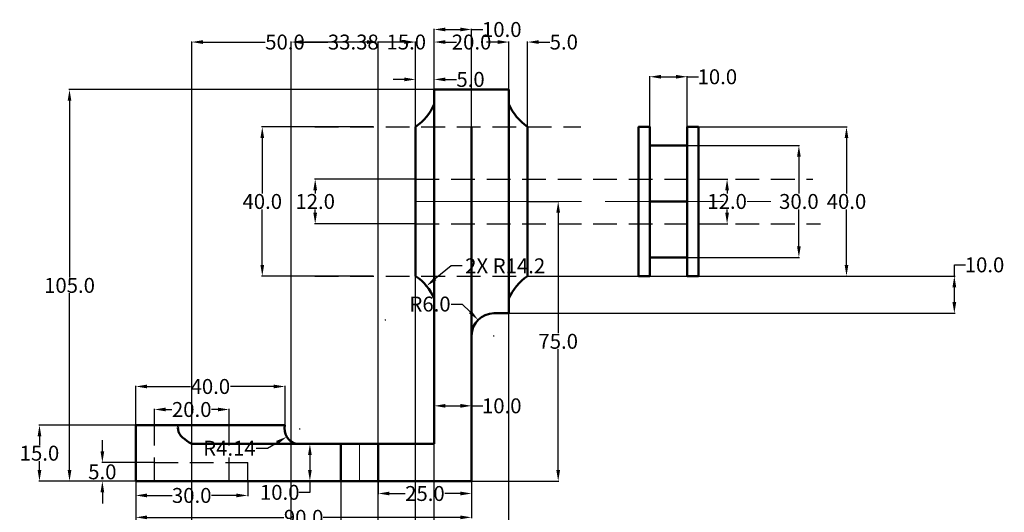
# Model space of a CAD drawing. Units: inches. Extents: x 846 to 1110, y 407 to 675.
# Tile 2 of 2: x 846 to 1110, y 542 to 675. Entities that reach past the tile are written whole.
import ezdxf

# ---------------------------------------------------------------- set-up
doc = ezdxf.new("R2010")
doc.units = ezdxf.units.IN
doc.header["$MEASUREMENT"] = 0
doc.linetypes.add('CENTER', pattern=[50.8, 31.75, -6.35, 6.35, -6.35])
doc.linetypes.add('HIDDEN', pattern=[9.525, 6.35, -3.175])
for name, color, linetype, lineweight in [('M-CNTR', 1, 'CENTER', 18), ('M-DIMS', 2, 'Continuous', 25), ('M-HIDN', 30, 'HIDDEN', 25), ('M-OUTL', 7, 'Continuous', 50)]:
    doc.layers.add(name, color=color, linetype=linetype, lineweight=lineweight)
doc.styles.get("Standard").update_dxf_attribs({"font": 'arial.ttf'})
doc.dimstyles.get("Standard").update_dxf_attribs({"dimtxt": 4, "dimasz": 3, "dimexe": 0.18, "dimexo": 0.0625, "dimgap": 0.09, "dimtad": 0, "dimtih": 1, "dimtoh": 1, "dimdec": 1, "dimzin": 0, "dimdsep": 46, "dimtxsty": 'Standard', "dimcen": 0.09, "dimadec": 0, "dimazin": 0, "dimtfac": 1, "dimtdec": 1, "dimtofl": 0, "dimtmove": 0, "dimatfit": 3, "dimfxl": 1, "dimtolj": 1, "dimtzin": 0, "dimarcsym": 0})

# ---------------------------------------------------------------- blocks, each defined once
blk = doc.blocks.new('*D1')
at = {"layer": 'Defpoints', "color": 0, "transparency": 16777216}
for p in [(902.2, 570.05), (882.2, 565.83), (902.2, 565.83)]:
    blk.add_point(p, dxfattribs=at)
at = {"layer": 'M-DIMS', "color": 0, "lineweight": -2, "transparency": 16777216}
for p, q in [((882.2, 565.9), (882.2, 570.23)), ((885.2, 570.05), (886.88, 570.05)), ((899.2, 570.05), (897.51, 570.05)), ((902.2, 565.9), (902.2, 570.23))]:
    blk.add_line(p, q, dxfattribs=at)
at = {"layer": 'M-DIMS', "color": 0, "transparency": 16777216}
for points in [[(885.2, 570.55), (885.2, 569.55), (882.2, 570.05)], [(899.2, 570.55), (899.2, 569.55), (902.2, 570.05)]]:
    blk.add_solid(points, dxfattribs=at)
at = {"layer": 'M-DIMS', "color": 0, "transparency": 16777216, "insert": (892.2, 570.05), "char_height": 4, "attachment_point": 5}
blk.add_mtext('\\A1;20.0', dxfattribs=at)
blk = doc.blocks.new('*D2')
at = {"layer": 'Defpoints', "color": 0, "transparency": 16777216}
for p in [(917.2, 576.22), (877.2, 565.83), (917.2, 565.83)]:
    blk.add_point(p, dxfattribs=at)
at = {"layer": 'M-DIMS', "color": 0, "lineweight": -2, "transparency": 16777216}
for p, q in [((877.2, 565.9), (877.2, 576.4)), ((880.2, 576.22), (891.84, 576.22)), ((914.2, 576.22), (902.56, 576.22)), ((917.2, 565.9), (917.2, 576.4))]:
    blk.add_line(p, q, dxfattribs=at)
at = {"layer": 'M-DIMS', "color": 0, "transparency": 16777216}
for points in [[(880.2, 576.72), (880.2, 575.72), (877.2, 576.22)], [(914.2, 576.72), (914.2, 575.72), (917.2, 576.22)]]:
    blk.add_solid(points, dxfattribs=at)
at = {"layer": 'M-DIMS', "color": 0, "transparency": 16777216, "insert": (897.2, 576.22), "char_height": 4, "attachment_point": 5}
blk.add_mtext('\\A1;40.0', dxfattribs=at)
blk = doc.blocks.new('*D3')
at = {"layer": 'Defpoints', "color": 0, "transparency": 16777216}
for p in [(877.2, 565.83), (851.4, 550.83), (877.2, 550.83)]:
    blk.add_point(p, dxfattribs=at)
at = {"layer": 'M-DIMS', "color": 0, "lineweight": -2, "transparency": 16777216}
for p, q in [((877.13, 565.83), (851.22, 565.83)), ((851.4, 562.83), (851.4, 560.47)), ((851.4, 553.83), (851.4, 556.2)), ((877.13, 550.83), (851.22, 550.83))]:
    blk.add_line(p, q, dxfattribs=at)
at = {"layer": 'M-DIMS', "color": 0, "transparency": 16777216}
for points in [[(850.9, 562.83), (851.9, 562.83), (851.4, 565.83)], [(850.9, 553.83), (851.9, 553.83), (851.4, 550.83)]]:
    blk.add_solid(points, dxfattribs=at)
at = {"layer": 'M-DIMS', "color": 0, "transparency": 16777216, "insert": (851.4, 558.33), "char_height": 4, "attachment_point": 5}
blk.add_mtext('\\A1;15.0', dxfattribs=at)
blk = doc.blocks.new('*D4')
at = {"layer": 'Defpoints', "color": 0, "transparency": 16777216}
for p in [(882.2, 555.83), (868.25, 550.83), (882.2, 550.83)]:
    blk.add_point(p, dxfattribs=at)
at = {"layer": 'M-DIMS', "color": 0, "lineweight": -2, "transparency": 16777216}
for p, q in [((868.25, 558.83), (868.25, 561.83)), ((882.13, 555.83), (868.07, 555.83)), ((882.13, 550.83), (868.07, 550.83)), ((868.25, 547.83), (868.25, 544.83))]:
    blk.add_line(p, q, dxfattribs=at)
at = {"layer": 'M-DIMS', "color": 0, "transparency": 16777216}
for points in [[(867.75, 558.83), (868.75, 558.83), (868.25, 555.83)], [(867.75, 547.83), (868.75, 547.83), (868.25, 550.83)]]:
    blk.add_solid(points, dxfattribs=at)
at = {"layer": 'M-DIMS', "color": 0, "transparency": 16777216, "insert": (868.25, 553.33), "char_height": 4, "attachment_point": 5}
blk.add_mtext('\\A1;5.0', dxfattribs=at)
blk = doc.blocks.new('*D5')
at = {"layer": 'Defpoints', "color": 0, "transparency": 16777216}
for p in [(877.2, 550.83), (907.2, 550.83), (907.2, 547)]:
    blk.add_point(p, dxfattribs=at)
at = {"layer": 'M-DIMS', "color": 0, "lineweight": -2, "transparency": 16777216}
for p, q in [((877.2, 550.77), (877.2, 546.82)), ((907.2, 550.77), (907.2, 546.82)), ((880.2, 547), (886.92, 547)), ((904.2, 547), (897.47, 547))]:
    blk.add_line(p, q, dxfattribs=at)
at = {"layer": 'M-DIMS', "color": 0, "transparency": 16777216}
for points in [[(880.2, 547.5), (880.2, 546.5), (877.2, 547)], [(904.2, 547.5), (904.2, 546.5), (907.2, 547)]]:
    blk.add_solid(points, dxfattribs=at)
at = {"layer": 'M-DIMS', "color": 0, "transparency": 16777216, "insert": (892.2, 547), "char_height": 4, "attachment_point": 5}
blk.add_mtext('\\A1;30.0', dxfattribs=at)
blk = doc.blocks.new('*D6')
at = {"layer": 'Defpoints', "color": 0, "transparency": 16777216}
for p in [(877.2, 550.83), (967.2, 550.83), (967.2, 541.12)]:
    blk.add_point(p, dxfattribs=at)
at = {"layer": 'M-DIMS', "color": 0, "lineweight": -2, "transparency": 16777216}
for p, q in [((877.2, 550.77), (877.2, 540.94)), ((967.2, 550.77), (967.2, 540.94)), ((880.2, 541.12), (916.92, 541.12)), ((964.2, 541.12), (927.47, 541.12))]:
    blk.add_line(p, q, dxfattribs=at)
at = {"layer": 'M-DIMS', "color": 0, "transparency": 16777216}
for points in [[(880.2, 541.62), (880.2, 540.62), (877.2, 541.12)], [(964.2, 541.62), (964.2, 540.62), (967.2, 541.12)]]:
    blk.add_solid(points, dxfattribs=at)
at = {"layer": 'M-DIMS', "color": 0, "transparency": 16777216, "insert": (922.2, 541.12), "char_height": 4, "attachment_point": 5}
blk.add_mtext('\\A1;90.0', dxfattribs=at)
blk = doc.blocks.new('*D7')
at = {"layer": 'Defpoints', "color": 0, "transparency": 16777216}
for p in [(924.94, 560.83), (923.87, 550.83), (924.94, 550.83)]:
    blk.add_point(p, dxfattribs=at)
at = {"layer": 'M-DIMS', "color": 0, "lineweight": -2, "transparency": 16777216}
for p, q in [((924.87, 560.83), (923.69, 560.83)), ((923.87, 557.83), (923.87, 553.83)), ((924.87, 550.83), (923.69, 550.83)), ((923.87, 550.83), (923.87, 547.83)), ((923.87, 547.83), (920.87, 547.83))]:
    blk.add_line(p, q, dxfattribs=at)
at = {"layer": 'M-DIMS', "color": 0, "transparency": 16777216}
for points in [[(923.37, 557.83), (924.37, 557.83), (923.87, 560.83)], [(923.37, 553.83), (924.37, 553.83), (923.87, 550.83)]]:
    blk.add_solid(points, dxfattribs=at)
at = {"layer": 'M-DIMS', "color": 0, "transparency": 16777216, "insert": (915.78, 547.83), "char_height": 4, "attachment_point": 5}
blk.add_mtext('\\A1;10.0', dxfattribs=at)
blk = doc.blocks.new('*D8')
at = {"layer": 'Defpoints', "color": 0, "transparency": 16777216}
for p in [(942.2, 550.83), (967.2, 550.83), (967.2, 547.52)]:
    blk.add_point(p, dxfattribs=at)
at = {"layer": 'M-DIMS', "color": 0, "lineweight": -2, "transparency": 16777216}
for p, q in [((942.2, 550.77), (942.2, 547.34)), ((967.2, 550.77), (967.2, 547.34)), ((945.2, 547.52), (949.38, 547.52)), ((964.2, 547.52), (960.01, 547.52))]:
    blk.add_line(p, q, dxfattribs=at)
at = {"layer": 'M-DIMS', "color": 0, "transparency": 16777216}
for points in [[(945.2, 548.02), (945.2, 547.02), (942.2, 547.52)], [(964.2, 548.02), (964.2, 547.02), (967.2, 547.52)]]:
    blk.add_solid(points, dxfattribs=at)
at = {"layer": 'M-DIMS', "color": 0, "transparency": 16777216, "insert": (954.7, 547.52), "char_height": 4, "attachment_point": 5}
blk.add_mtext('\\A1;25.0', dxfattribs=at)
blk = doc.blocks.new('*D9')
at = {"layer": 'Defpoints', "color": 0, "transparency": 16777216}
for p in [(940.93, 645.83), (911.11, 605.83), (940.93, 605.83)]:
    blk.add_point(p, dxfattribs=at)
at = {"layer": 'M-DIMS', "color": 0, "lineweight": -2, "transparency": 16777216}
for p, q in [((940.87, 645.83), (910.93, 645.83)), ((911.11, 642.83), (911.11, 627.97)), ((911.11, 608.83), (911.11, 623.7)), ((940.87, 605.83), (910.93, 605.83))]:
    blk.add_line(p, q, dxfattribs=at)
at = {"layer": 'M-DIMS', "color": 0, "transparency": 16777216}
for points in [[(910.61, 642.83), (911.61, 642.83), (911.11, 645.83)], [(910.61, 608.83), (911.61, 608.83), (911.11, 605.83)]]:
    blk.add_solid(points, dxfattribs=at)
at = {"layer": 'M-DIMS', "color": 0, "transparency": 16777216, "insert": (911.11, 625.83), "char_height": 4, "attachment_point": 5}
blk.add_mtext('\\A1;40.0', dxfattribs=at)
blk = doc.blocks.new('*D10')
at = {"layer": 'Defpoints', "color": 0, "transparency": 16777216}
for p in [(952.2, 631.83), (925.29, 619.83), (952.2, 619.83)]:
    blk.add_point(p, dxfattribs=at)
at = {"layer": 'M-DIMS', "color": 0, "lineweight": -2, "transparency": 16777216}
for p, q in [((952.13, 631.83), (925.11, 631.83)), ((925.29, 628.83), (925.29, 627.97)), ((925.29, 622.83), (925.29, 623.7)), ((952.13, 619.83), (925.11, 619.83))]:
    blk.add_line(p, q, dxfattribs=at)
at = {"layer": 'M-DIMS', "color": 0, "transparency": 16777216}
for points in [[(924.79, 628.83), (925.79, 628.83), (925.29, 631.83)], [(924.79, 622.83), (925.79, 622.83), (925.29, 619.83)]]:
    blk.add_solid(points, dxfattribs=at)
at = {"layer": 'M-DIMS', "color": 0, "transparency": 16777216, "insert": (925.29, 625.83), "char_height": 4, "attachment_point": 5}
blk.add_mtext('\\A1;12.0', dxfattribs=at)
blk = doc.blocks.new('*D11')
at = {"layer": 'Defpoints', "color": 0, "transparency": 16777216}
for p in [(1024.98, 659.27), (1014.98, 625.83), (1024.98, 625.83)]:
    blk.add_point(p, dxfattribs=at)
at = {"layer": 'M-DIMS', "color": 0, "lineweight": -2, "transparency": 16777216}
for p, q in [((1014.98, 625.9), (1014.98, 659.45)), ((1017.98, 659.27), (1021.98, 659.27)), ((1024.98, 625.9), (1024.98, 659.45)), ((1024.98, 659.27), (1027.98, 659.27))]:
    blk.add_line(p, q, dxfattribs=at)
at = {"layer": 'M-DIMS', "color": 0, "transparency": 16777216}
for points in [[(1017.98, 659.77), (1017.98, 658.77), (1014.98, 659.27)], [(1021.98, 659.77), (1021.98, 658.77), (1024.98, 659.27)]]:
    blk.add_solid(points, dxfattribs=at)
at = {"layer": 'M-DIMS', "color": 0, "transparency": 16777216, "insert": (1033.07, 659.27), "char_height": 4, "attachment_point": 5}
blk.add_mtext('\\A1;10.0', dxfattribs=at)
blk = doc.blocks.new('*D12')
at = {"layer": 'Defpoints', "color": 0, "transparency": 16777216}
for p in [(1024.98, 640.83), (1024.98, 610.83), (1054.92, 610.83)]:
    blk.add_point(p, dxfattribs=at)
at = {"layer": 'M-DIMS', "color": 0, "lineweight": -2, "transparency": 16777216}
for p, q in [((1025.04, 640.83), (1055.1, 640.83)), ((1054.92, 637.83), (1054.92, 627.97)), ((1054.92, 613.83), (1054.92, 623.7)), ((1025.04, 610.83), (1055.1, 610.83))]:
    blk.add_line(p, q, dxfattribs=at)
at = {"layer": 'M-DIMS', "color": 0, "transparency": 16777216}
for points in [[(1054.42, 637.83), (1055.42, 637.83), (1054.92, 640.83)], [(1054.42, 613.83), (1055.42, 613.83), (1054.92, 610.83)]]:
    blk.add_solid(points, dxfattribs=at)
at = {"layer": 'M-DIMS', "color": 0, "transparency": 16777216, "insert": (1054.92, 625.83), "char_height": 4, "attachment_point": 5}
blk.add_mtext('\\A1;30.0', dxfattribs=at)
blk = doc.blocks.new('*D13')
at = {"layer": 'Defpoints', "color": 0, "transparency": 16777216}
for p in [(1031.16, 631.83), (1031.16, 619.83), (1035.68, 619.83)]:
    blk.add_point(p, dxfattribs=at)
at = {"layer": 'M-DIMS', "color": 0, "lineweight": -2, "transparency": 16777216}
for p, q in [((1031.22, 631.83), (1035.86, 631.83)), ((1035.68, 628.83), (1035.68, 627.97)), ((1035.68, 622.83), (1035.68, 623.7)), ((1031.22, 619.83), (1035.86, 619.83))]:
    blk.add_line(p, q, dxfattribs=at)
at = {"layer": 'M-DIMS', "color": 0, "transparency": 16777216}
for points in [[(1035.18, 628.83), (1036.18, 628.83), (1035.68, 631.83)], [(1035.18, 622.83), (1036.18, 622.83), (1035.68, 619.83)]]:
    blk.add_solid(points, dxfattribs=at)
at = {"layer": 'M-DIMS', "color": 0, "transparency": 16777216, "insert": (1035.68, 625.83), "char_height": 4, "attachment_point": 5}
blk.add_mtext('\\A1;12.0', dxfattribs=at)
blk = doc.blocks.new('*D14')
at = {"layer": 'Defpoints', "color": 0, "transparency": 16777216}
for p in [(1027.98, 645.83), (1027.98, 605.83), (1067.68, 605.83)]:
    blk.add_point(p, dxfattribs=at)
at = {"layer": 'M-DIMS', "color": 0, "lineweight": -2, "transparency": 16777216}
for p, q in [((1028.04, 645.83), (1067.86, 645.83)), ((1067.68, 642.83), (1067.68, 627.97)), ((1067.68, 608.83), (1067.68, 623.7)), ((1028.04, 605.83), (1067.86, 605.83))]:
    blk.add_line(p, q, dxfattribs=at)
at = {"layer": 'M-DIMS', "color": 0, "transparency": 16777216}
for points in [[(1067.18, 642.83), (1068.18, 642.83), (1067.68, 645.83)], [(1067.18, 608.83), (1068.18, 608.83), (1067.68, 605.83)]]:
    blk.add_solid(points, dxfattribs=at)
at = {"layer": 'M-DIMS', "color": 0, "transparency": 16777216, "insert": (1067.68, 625.83), "char_height": 4, "attachment_point": 5}
blk.add_mtext('\\A1;40.0', dxfattribs=at)
blk = doc.blocks.new('*D15')
at = {"layer": 'Defpoints', "color": 0, "transparency": 16777216}
for p in [(957.2, 658.56), (952.2, 645.83), (957.2, 645.83)]:
    blk.add_point(p, dxfattribs=at)
at = {"layer": 'M-DIMS', "color": 0, "lineweight": -2, "transparency": 16777216}
for p, q in [((949.2, 658.56), (946.2, 658.56)), ((952.2, 645.9), (952.2, 658.74)), ((957.2, 645.9), (957.2, 658.74)), ((960.2, 658.56), (963.2, 658.56))]:
    blk.add_line(p, q, dxfattribs=at)
at = {"layer": 'M-DIMS', "color": 0, "transparency": 16777216}
for points in [[(949.2, 659.06), (949.2, 658.06), (952.2, 658.56)], [(960.2, 659.06), (960.2, 658.06), (957.2, 658.56)]]:
    blk.add_solid(points, dxfattribs=at)
at = {"layer": 'M-DIMS', "color": 0, "transparency": 16777216, "insert": (966.92, 658.56), "char_height": 4, "attachment_point": 5}
blk.add_mtext('\\A1;5.0', dxfattribs=at)
blk = doc.blocks.new('*D16')
at = {"layer": 'Defpoints', "color": 0, "transparency": 16777216}
for p in [(967.2, 671.95), (957.2, 645.83), (967.2, 645.83)]:
    blk.add_point(p, dxfattribs=at)
at = {"layer": 'M-DIMS', "color": 0, "lineweight": -2, "transparency": 16777216}
for p, q in [((957.2, 645.9), (957.2, 672.13)), ((960.2, 671.95), (964.2, 671.95)), ((967.2, 645.9), (967.2, 672.13)), ((967.2, 671.95), (970.2, 671.95))]:
    blk.add_line(p, q, dxfattribs=at)
at = {"layer": 'M-DIMS', "color": 0, "transparency": 16777216}
for points in [[(960.2, 672.45), (960.2, 671.45), (957.2, 671.95)], [(964.2, 672.45), (964.2, 671.45), (967.2, 671.95)]]:
    blk.add_solid(points, dxfattribs=at)
at = {"layer": 'M-DIMS', "color": 0, "transparency": 16777216, "insert": (975.29, 671.95), "char_height": 4, "attachment_point": 5}
blk.add_mtext('\\A1;10.0', dxfattribs=at)
blk = doc.blocks.new('*D17')
at = {"layer": 'Defpoints', "color": 0, "transparency": 16777216}
for p in [(982.2, 625.83), (967.2, 550.83), (990.42, 550.83)]:
    blk.add_point(p, dxfattribs=at)
at = {"layer": 'M-DIMS', "color": 0, "lineweight": -2, "transparency": 16777216}
for p, q in [((982.26, 625.83), (990.6, 625.83)), ((990.42, 622.83), (990.42, 590.47)), ((990.42, 553.83), (990.42, 586.2)), ((967.26, 550.83), (990.6, 550.83))]:
    blk.add_line(p, q, dxfattribs=at)
at = {"layer": 'M-DIMS', "color": 0, "transparency": 16777216}
for points in [[(989.92, 622.83), (990.92, 622.83), (990.42, 625.83)], [(989.92, 553.83), (990.92, 553.83), (990.42, 550.83)]]:
    blk.add_solid(points, dxfattribs=at)
at = {"layer": 'M-DIMS', "color": 0, "transparency": 16777216, "insert": (990.42, 588.33), "char_height": 4, "attachment_point": 5}
blk.add_mtext('\\A1;75.0', dxfattribs=at)
blk = doc.blocks.new('*D21')
at = {"layer": 'Defpoints', "color": 0, "transparency": 16777216}
for p in [(967.2, 571.03), (957.2, 569.71), (967.2, 569.71)]:
    blk.add_point(p, dxfattribs=at)
at = {"layer": 'M-DIMS', "color": 0, "lineweight": -2, "transparency": 16777216}
for p, q in [((957.2, 569.77), (957.2, 571.21)), ((960.2, 571.03), (964.2, 571.03)), ((967.2, 569.77), (967.2, 571.21)), ((967.2, 571.03), (970.2, 571.03))]:
    blk.add_line(p, q, dxfattribs=at)
at = {"layer": 'M-DIMS', "color": 0, "transparency": 16777216}
for points in [[(960.2, 571.53), (960.2, 570.53), (957.2, 571.03)], [(964.2, 571.53), (964.2, 570.53), (967.2, 571.03)]]:
    blk.add_solid(points, dxfattribs=at)
at = {"layer": 'M-DIMS', "color": 0, "transparency": 16777216, "insert": (975.29, 571.03), "char_height": 4, "attachment_point": 5}
blk.add_mtext('\\A1;10.0', dxfattribs=at)
blk = doc.blocks.new('*D22')
at = {"layer": 'Defpoints', "color": 0, "transparency": 16777216}
for p in [(942.2, 668.58), (942.2, 512.61), (892.2, 467.61)]:
    blk.add_point(p, dxfattribs=at)
at = {"layer": 'M-DIMS', "color": 0, "lineweight": -2, "transparency": 16777216}
for p, q in [((892.2, 467.67), (892.2, 668.76)), ((895.2, 668.58), (911.92, 668.58)), ((939.2, 668.58), (922.47, 668.58)), ((942.2, 512.67), (942.2, 668.76))]:
    blk.add_line(p, q, dxfattribs=at)
at = {"layer": 'M-DIMS', "color": 0, "transparency": 16777216}
for points in [[(895.2, 669.08), (895.2, 668.08), (892.2, 668.58)], [(939.2, 669.08), (939.2, 668.08), (942.2, 668.58)]]:
    blk.add_solid(points, dxfattribs=at)
at = {"layer": 'M-DIMS', "color": 0, "transparency": 16777216, "insert": (917.2, 668.58), "char_height": 4, "attachment_point": 5}
blk.add_mtext('\\A1;50.0', dxfattribs=at)
blk = doc.blocks.new('*D23')
at = {"layer": 'Defpoints', "color": 0, "transparency": 16777216}
for p in [(957.196639, 668.584955), (942.196639, 512.605991), (957.196639, 512.605991)]:
    blk.add_point(p, dxfattribs=at)
at = {"layer": 'M-DIMS', "color": 0, "lineweight": -2, "transparency": 16777216}
for p, q in [((939.196639, 668.584955), (936.196639, 668.584955)), ((942.196639, 512.668491), (942.196639, 668.764955)), ((957.196639, 512.668491), (957.196639, 668.764955)), ((960.196639, 668.584955), (963.196639, 668.584955))]:
    blk.add_line(p, q, dxfattribs=at)
at = {"layer": 'M-DIMS', "color": 0, "transparency": 16777216}
for points in [[(939.196639, 669.084955), (939.196639, 668.084955), (942.196639, 668.584955)], [(960.196639, 669.084955), (960.196639, 668.084955), (957.196639, 668.584955)]]:
    blk.add_solid(points, dxfattribs=at)
at = {"layer": 'M-DIMS', "color": 0, "transparency": 16777216, "insert": (949.696639, 668.584955), "char_height": 4, "attachment_point": 5}
blk.add_mtext('\\A1;15.0', dxfattribs=at)
blk = doc.blocks.new('*D24')
at = {"layer": 'Defpoints', "color": 0, "transparency": 16777216}
for p in [(977.2, 668.58), (957.2, 512.61), (977.2, 512.61)]:
    blk.add_point(p, dxfattribs=at)
at = {"layer": 'M-DIMS', "color": 0, "lineweight": -2, "transparency": 16777216}
for p, q in [((957.2, 512.67), (957.2, 668.76)), ((960.2, 668.58), (961.88, 668.58)), ((974.2, 668.58), (972.51, 668.58)), ((977.2, 512.67), (977.2, 668.76))]:
    blk.add_line(p, q, dxfattribs=at)
at = {"layer": 'M-DIMS', "color": 0, "transparency": 16777216}
for points in [[(960.2, 669.08), (960.2, 668.08), (957.2, 668.58)], [(974.2, 669.08), (974.2, 668.08), (977.2, 668.58)]]:
    blk.add_solid(points, dxfattribs=at)
at = {"layer": 'M-DIMS', "color": 0, "transparency": 16777216, "insert": (967.2, 668.58), "char_height": 4, "attachment_point": 5}
blk.add_mtext('\\A1;20.0', dxfattribs=at)
blk = doc.blocks.new('*D26')
at = {"layer": 'Defpoints', "color": 0, "transparency": 16777216}
for p in [(952.2, 668.58), (918.81, 472.61), (952.2, 472.61)]:
    blk.add_point(p, dxfattribs=at)
at = {"layer": 'M-DIMS', "color": 0, "lineweight": -2, "transparency": 16777216}
for p, q in [((918.81, 472.67), (918.81, 668.76)), ((921.81, 668.58), (928.66, 668.58)), ((949.2, 668.58), (942.35, 668.58)), ((952.2, 472.67), (952.2, 668.76))]:
    blk.add_line(p, q, dxfattribs=at)
at = {"layer": 'M-DIMS', "color": 0, "transparency": 16777216}
for points in [[(921.81, 669.08), (921.81, 668.08), (918.81, 668.58)], [(949.2, 669.08), (949.2, 668.08), (952.2, 668.58)]]:
    blk.add_solid(points, dxfattribs=at)
at = {"layer": 'M-DIMS', "color": 0, "transparency": 16777216, "insert": (935.51, 668.58), "char_height": 4, "attachment_point": 5}
blk.add_mtext('\\A1;33.38', dxfattribs=at)
blk = doc.blocks.new('*D30')
at = {"layer": 'Defpoints', "color": 0, "transparency": 16777216}
for p in [(957.2, 655.83), (859.45, 550.83), (967.2, 550.83)]:
    blk.add_point(p, dxfattribs=at)
at = {"layer": 'M-DIMS', "color": 0, "lineweight": -2, "transparency": 16777216}
for p, q in [((957.13, 655.83), (859.27, 655.83)), ((859.45, 652.83), (859.45, 605.47)), ((859.45, 553.83), (859.45, 601.2)), ((967.13, 550.83), (859.27, 550.83))]:
    blk.add_line(p, q, dxfattribs=at)
at = {"layer": 'M-DIMS', "color": 0, "transparency": 16777216}
for points in [[(858.95, 652.83), (859.95, 652.83), (859.45, 655.83)], [(858.95, 553.83), (859.95, 553.83), (859.45, 550.83)]]:
    blk.add_solid(points, dxfattribs=at)
at = {"layer": 'M-DIMS', "color": 0, "transparency": 16777216, "insert": (859.45, 603.33), "char_height": 4, "attachment_point": 5}
blk.add_mtext('\\A1;105.0', dxfattribs=at)
blk = doc.blocks.new('*D31')
at = {"layer": 'Defpoints', "color": 0, "transparency": 16777216}
for p in [(982.196639, 605.834955), (1096.581479, 605.834955), (977.196639, 595.834955)]:
    blk.add_point(p, dxfattribs=at)
at = {"layer": 'M-DIMS', "color": 0, "lineweight": -2, "transparency": 16777216}
for p, q in [((1096.581479, 605.834955), (1096.581479, 608.834955)), ((1096.581479, 608.834955), (1099.581479, 608.834955)), ((982.259139, 605.834955), (1096.761479, 605.834955)), ((1096.581479, 598.834955), (1096.581479, 602.834955)), ((977.259139, 595.834955), (1096.761479, 595.834955))]:
    blk.add_line(p, q, dxfattribs=at)
at = {"layer": 'M-DIMS', "color": 0, "transparency": 16777216}
for points in [[(1096.081479, 602.834955), (1097.081479, 602.834955), (1096.581479, 605.834955)], [(1096.081479, 598.834955), (1097.081479, 598.834955), (1096.581479, 595.834955)]]:
    blk.add_solid(points, dxfattribs=at)
at = {"layer": 'M-DIMS', "color": 0, "transparency": 16777216, "insert": (1104.671479, 608.834955), "char_height": 4, "attachment_point": 5}
blk.add_mtext('\\A1;10.0', dxfattribs=at)
blk = doc.blocks.new('*D32')
at = {"layer": 'Defpoints', "color": 0, "transparency": 16777216}
for p in [(977.2, 668.58), (957.2, 655.83), (977.2, 655.83)]:
    blk.add_point(p, dxfattribs=at)
at = {"layer": 'M-DIMS', "color": 0, "lineweight": -2, "transparency": 16777216}
for p, q in [((957.2, 655.9), (957.2, 668.76)), ((960.2, 668.58), (961.88, 668.58)), ((974.2, 668.58), (972.51, 668.58)), ((977.2, 655.9), (977.2, 668.76))]:
    blk.add_line(p, q, dxfattribs=at)
at = {"layer": 'M-DIMS', "color": 0, "transparency": 16777216}
for points in [[(960.2, 669.08), (960.2, 668.08), (957.2, 668.58)], [(974.2, 669.08), (974.2, 668.08), (977.2, 668.58)]]:
    blk.add_solid(points, dxfattribs=at)
at = {"layer": 'M-DIMS', "color": 0, "transparency": 16777216, "insert": (967.2, 668.58), "char_height": 4, "attachment_point": 5}
blk.add_mtext('\\A1;20.0', dxfattribs=at)
blk = doc.blocks.new('*D33')
at = {"layer": 'Defpoints', "color": 0, "transparency": 16777216}
for p in [(982.2, 668.58), (977.2, 655.83), (982.2, 645.83)]:
    blk.add_point(p, dxfattribs=at)
at = {"layer": 'M-DIMS', "color": 0, "lineweight": -2, "transparency": 16777216}
for p, q in [((974.2, 668.58), (971.2, 668.58)), ((977.2, 655.9), (977.2, 668.76)), ((982.2, 645.9), (982.2, 668.76)), ((985.2, 668.58), (988.2, 668.58))]:
    blk.add_line(p, q, dxfattribs=at)
at = {"layer": 'M-DIMS', "color": 0, "transparency": 16777216}
for points in [[(974.2, 669.08), (974.2, 668.08), (977.2, 668.58)], [(985.2, 669.08), (985.2, 668.08), (982.2, 668.58)]]:
    blk.add_solid(points, dxfattribs=at)
at = {"layer": 'M-DIMS', "color": 0, "transparency": 16777216, "insert": (991.92, 668.58), "char_height": 4, "attachment_point": 5}
blk.add_mtext('\\A1;5.0', dxfattribs=at)
blk = doc.blocks.new('*D34')
at = {"layer": 'Defpoints', "color": 0, "transparency": 16777216}
for p in [(877.2, 550.83), (932.2, 550.83), (932.2, 409.86)]:
    blk.add_point(p, dxfattribs=at)
at = {"layer": 'M-DIMS', "color": 0, "lineweight": -2, "transparency": 16777216}
for p, q in [((877.2, 550.77), (877.2, 409.68)), ((932.2, 550.77), (932.2, 409.68)), ((880.2, 409.86), (899.42, 409.86)), ((929.2, 409.86), (909.97, 409.86))]:
    blk.add_line(p, q, dxfattribs=at)
at = {"layer": 'M-DIMS', "color": 0, "transparency": 16777216}
for points in [[(880.2, 410.36), (880.2, 409.36), (877.2, 409.86)], [(929.2, 410.36), (929.2, 409.36), (932.2, 409.86)]]:
    blk.add_solid(points, dxfattribs=at)
at = {"layer": 'M-DIMS', "color": 0, "transparency": 16777216, "insert": (904.7, 409.86), "char_height": 4, "attachment_point": 5}
blk.add_mtext('\\A1;55.0', dxfattribs=at)
blk = doc.blocks.new('*D44')
at = {"layer": 'Defpoints', "color": 0, "transparency": 16777216}
for p in [(955.12, 603.15), (944.17, 594.12)]:
    blk.add_point(p, dxfattribs=at)
at = {"layer": 'M-DIMS', "color": 0, "lineweight": -2, "transparency": 16777216}
for p, q in [((961.7, 608.57), (957.44, 605.06)), ((964.7, 608.57), (961.7, 608.57)), ((944.08, 594.12), (944.26, 594.12)), ((944.17, 594.03), (944.17, 594.21))]:
    blk.add_line(p, q, dxfattribs=at)
at = {"layer": 'M-DIMS', "color": 0, "transparency": 16777216}
blk.add_solid([(957.12, 605.45), (957.76, 604.68), (955.12, 603.15)], dxfattribs=at)
at = {"layer": 'M-DIMS', "color": 0, "transparency": 16777216, "insert": (976.21, 608.57), "char_height": 4, "attachment_point": 5}
blk.add_mtext('\\A1;2X R14.2', dxfattribs=at)
blk = doc.blocks.new('*D45')
at = {"layer": 'Defpoints', "color": 0, "transparency": 16777216}
for p in [(968.95, 594.08), (973.2, 589.83)]:
    blk.add_point(p, dxfattribs=at)
at = {"layer": 'M-DIMS', "color": 0, "lineweight": -2, "transparency": 16777216}
for p, q in [((961.71, 598.32), (964.71, 598.32)), ((964.71, 598.32), (966.83, 596.2)), ((973.11, 589.83), (973.29, 589.83)), ((973.2, 589.74), (973.2, 589.92))]:
    blk.add_line(p, q, dxfattribs=at)
at = {"layer": 'M-DIMS', "color": 0, "transparency": 16777216}
blk.add_solid([(967.19, 596.55), (966.48, 595.85), (968.95, 594.08)], dxfattribs=at)
at = {"layer": 'M-DIMS', "color": 0, "transparency": 16777216, "insert": (956.07, 598.32), "char_height": 4, "attachment_point": 5}
blk.add_mtext('\\A1;R6.0', dxfattribs=at)
blk = doc.blocks.new('*D46')
at = {"layer": 'Defpoints', "color": 0, "transparency": 16777216}
for p in [(921.21, 564.84), (917.65, 562.72)]:
    blk.add_point(p, dxfattribs=at)
at = {"layer": 'M-DIMS', "color": 0, "lineweight": -2, "transparency": 16777216}
for p, q in [((921.12, 564.84), (921.3, 564.84)), ((921.21, 564.75), (921.21, 564.93)), ((909.5, 559.66), (912.5, 559.66)), ((912.5, 559.66), (915.08, 561.19))]:
    blk.add_line(p, q, dxfattribs=at)
at = {"layer": 'M-DIMS', "color": 0, "transparency": 16777216}
blk.add_solid([(914.82, 561.62), (915.33, 560.76), (917.65, 562.72)], dxfattribs=at)
at = {"layer": 'M-DIMS', "color": 0, "transparency": 16777216, "insert": (902.31, 559.66), "char_height": 4, "attachment_point": 5}
blk.add_mtext('\\A1;R4.14', dxfattribs=at)

msp = doc.modelspace()

# ---------------------------------------------------------------- linework, layer by layer
at = {"layer": 'M-CNTR'}
for p, q in [((952.1966, 625.835), (1049.7896, 625.835)), ((892.1966, 462.3642), (892.1966, 565.835)), ((937.1966, 550.835), (937.1966, 560.835))]:
    msp.add_line(p, q, dxfattribs=at)
at = {"layer": 'M-HIDN'}
for p, q in [((925.1611, 645.835), (996.4424, 645.835)), ((952.1966, 631.835), (1058.617, 631.835)), ((952.1966, 619.835), (1060.7178, 619.835)), ((925.1611, 605.835), (996.4424, 605.835)), ((882.1966, 550.835), (882.1966, 565.835)), ((902.1966, 550.835), (902.1966, 565.835)), ((882.1966, 555.835), (907.1966, 555.835)), ((907.1966, 550.835), (907.1966, 555.835))]:
    msp.add_line(p, q, dxfattribs=at)
at = {"layer": 'M-OUTL'}
for p, q in [((957.1966, 560.835), (957.1966, 655.835)), ((957.1966, 655.835), (977.1966, 655.835)), ((977.1966, 595.835), (977.1966, 655.835)), ((952.1966, 605.835), (952.1966, 645.835)), ((967.1966, 550.835), (967.1966, 645.835)), ((982.1966, 605.835), (982.1966, 645.835)), ((1014.9804, 640.835), (1024.9804, 640.835)), ((1014.9804, 625.835), (1024.9804, 625.835)), ((1014.9804, 610.835), (1024.9804, 610.835)), ((973.1966, 595.835), (977.1966, 595.835)), ((877.1966, 550.835), (877.1966, 565.835)), ((877.1966, 565.835), (917.1966, 565.835)), ((892.1966, 560.835), (957.1966, 560.835)), ((932.1966, 550.835), (932.1966, 560.835)), ((942.1966, 550.835), (942.1966, 560.835)), ((877.1966, 550.835), (967.1966, 550.835))]:
    msp.add_line(p, q, dxfattribs=at)
for points in [[(1014.9804, 605.835), (1014.9804, 645.835), (1011.9804, 645.835), (1011.9804, 605.835)], [(1027.9804, 605.835), (1027.9804, 645.835), (1024.9804, 645.835), (1024.9804, 605.835)]]:
    msp.add_lwpolyline(points, close=True, dxfattribs=at)
for centre, radius, start, end in [((944.1657, 657.5461), 14.2002, 304.440343, 336.585666), ((990.2275, 657.5461), 14.2002, 203.414334, 235.559657), ((944.1657, 594.1238), 14.2002, 23.414334, 55.559657), ((990.2275, 594.1238), 14.2002, 124.440343, 156.585666), ((973.1966, 589.835), 6, 90, 180), ((921.211, 564.8374), 4.1365, 166.044289, 255.372624)]:
    msp.add_arc(centre, radius, start, end, dxfattribs=at)
msp.add_open_spline([(892.1966, 560.835), (890.4461, 561.9102), (888.4305, 563.1483), (888.5229, 565.2271), (888.535, 565.5004)], degree=3, knots=[0, 0, 0, 0, 5.32046797, 6.12583745, 6.12583745, 6.12583745, 6.12583745], dxfattribs=at)

# ---------------------------------------------------------------- dimensions: what is measured, and where the dimension line sits
at = {"layer": 'M-DIMS'}
for base, p1, p2, override, picture, middle in [((967.1966, 671.954), (957.1966, 645.835), (967.1966, 645.835), {"dimclrd": 0, "dimclre": 0, "dimclrt": 0}, '*D16', (975.2866, 671.954)), ((942.1966, 668.585), (892.1966, 467.606), (942.1966, 512.606), {"dimdec": 1, "dimlfac": 1, "dimrnd": 0, "dimzin": 0, "dimdsep": 46, "dimlunit": 2}, '*D22', (917.1966, 668.585)), ((952.1966, 668.585), (918.8141, 472.606), (952.1966, 472.606), {"dimdec": 2, "dimlfac": 1, "dimrnd": 0, "dimzin": 0, "dimdsep": 46, "dimlunit": 2}, '*D26', (935.5054, 668.585)), ((957.1966, 668.585), (942.1966, 512.606), (957.1966, 512.606), {"dimdec": 1, "dimlfac": 1, "dimrnd": 0, "dimzin": 0, "dimdsep": 46, "dimlunit": 2}, '*D23', (949.6966, 668.585)), ((977.1966, 668.585), (957.1966, 512.606), (977.1966, 512.606), {"dimdec": 1, "dimlfac": 1, "dimrnd": 0, "dimzin": 0, "dimdsep": 46, "dimlunit": 2}, '*D24', (967.1966, 668.585)), ((977.1966, 668.585), (957.1966, 655.835), (977.1966, 655.835), {"dimdec": 1, "dimlfac": 1, "dimrnd": 0, "dimzin": 0, "dimdsep": 46, "dimlunit": 2}, '*D32', (967.1966, 668.585)), ((982.1966, 668.585), (977.1966, 655.835), (982.1966, 645.835), {"dimdec": 1, "dimlfac": 1, "dimrnd": 0, "dimzin": 0, "dimdsep": 46, "dimlunit": 2}, '*D33', (991.921, 668.585)), ((957.1966, 658.5581), (952.1966, 645.835), (957.1966, 645.835), {"dimclrd": 0, "dimclre": 0, "dimclrt": 0}, '*D15', (966.921, 658.5581)), ((1024.9804, 659.2682), (1014.9804, 625.835), (1024.9804, 625.835), {"dimclrd": 0, "dimclre": 0, "dimclrt": 0}, '*D11', (1033.0704, 659.2682)), ((917.1966, 576.2178), (877.1966, 565.835), (917.1966, 565.835), {"dimclrd": 0, "dimclre": 0, "dimclrt": 0}, '*D2', (897.1966, 576.2178)), ((902.1966, 570.0517), (882.1966, 565.835), (902.1966, 565.835), {"dimclrd": 0, "dimclre": 0, "dimclrt": 0}, '*D1', (892.1966, 570.0517)), ((967.1966, 571.0288), (957.1966, 569.7121), (967.1966, 569.7121), {"dimclrd": 0, "dimclre": 0, "dimclrt": 0}, '*D21', (975.2866, 571.0288)), ((907.1966, 546.9977), (877.1966, 550.835), (907.1966, 550.835), {"dimclrd": 0, "dimclre": 0, "dimclrt": 0}, '*D5', (892.1966, 546.9977)), ((967.1966, 541.1223), (877.1966, 550.835), (967.1966, 550.835), {"dimclrd": 0, "dimclre": 0, "dimclrt": 0}, '*D6', (922.1966, 541.1223)), ((932.1966, 409.856), (877.1966, 550.835), (932.1966, 550.835), {"dimdec": 1, "dimlfac": 1, "dimrnd": 0, "dimzin": 0, "dimdsep": 46, "dimlunit": 2}, '*D34', (904.6966, 409.856)), ((967.1966, 547.5178), (942.1966, 550.835), (967.1966, 550.835), {"dimclrd": 0, "dimclre": 0, "dimclrt": 0}, '*D8', (954.6966, 547.5178))]:
    dim = msp.add_linear_dim(base=base, p1=p1, p2=p2, dimstyle='Standard', override=override, dxfattribs=at)
    dim.commit()
    dim.dimension.update_dxf_attribs({"geometry": picture, "text_midpoint": middle})
for base, p1, p2, override, picture, middle in [((859.4466, 550.835), (957.1966, 655.835), (967.1966, 550.835), {"dimdec": 1, "dimlfac": 1, "dimrnd": 0, "dimzin": 0, "dimdsep": 46, "dimlunit": 2}, '*D30', (859.4466, 603.335)), ((911.1144, 605.835), (940.9322, 645.835), (940.9322, 605.835), {"dimclrd": 0, "dimclre": 0, "dimclrt": 0}, '*D9', (911.1144, 625.835)), ((1067.6823, 605.835), (1027.9804, 645.835), (1027.9804, 605.835), {"dimclrd": 0, "dimclre": 0, "dimclrt": 0}, '*D14', (1067.6823, 625.835)), ((1054.9157, 610.835), (1024.9804, 640.835), (1024.9804, 610.835), {"dimclrd": 0, "dimclre": 0, "dimclrt": 0}, '*D12', (1054.9157, 625.835)), ((925.2895, 619.835), (952.1966, 631.835), (952.1966, 619.835), {"dimclrd": 0, "dimclre": 0, "dimclrt": 0}, '*D10', (925.2895, 625.835)), ((1035.6849, 619.835), (1031.16, 631.835), (1031.16, 619.835), {"dimclrd": 0, "dimclre": 0, "dimclrt": 0}, '*D13', (1035.6849, 625.835)), ((990.4153, 550.835), (982.1966, 625.835), (967.1966, 550.835), {"dimclrd": 0, "dimclre": 0, "dimclrt": 0}, '*D17', (990.4153, 588.335)), ((1096.5815, 605.835), (977.1966, 595.835), (982.1966, 605.835), {"dimdec": 1, "dimlfac": 1, "dimrnd": 0, "dimzin": 0, "dimdsep": 46, "dimlunit": 2}, '*D31', (1104.6715, 608.835)), ((851.3992, 550.835), (877.1966, 565.835), (877.1966, 550.835), {"dimclrd": 0, "dimclre": 0, "dimclrt": 0}, '*D3', (851.3992, 558.335)), ((868.2459, 550.835), (882.1966, 555.835), (882.1966, 550.835), {"dimclrd": 0, "dimclre": 0, "dimclrt": 0}, '*D4', (868.2459, 553.335)), ((923.8678, 550.835), (924.9374, 560.835), (924.9374, 550.835), {"dimclrd": 0, "dimclre": 0, "dimclrt": 0}, '*D7', (915.7778, 547.835))]:
    dim = msp.add_linear_dim(base=base, p1=p1, p2=p2, angle=90, dimstyle='Standard', override=override, dxfattribs=at)
    dim.commit()
    dim.dimension.update_dxf_attribs({"geometry": picture, "text_midpoint": middle})
dim = msp.add_radius_dim(center=(944.1657, 594.1238), mpoint=(955.1249, 603.1539), text='2X <>', dimstyle='Standard', override={"dimdec": 1, "dimlfac": 1, "dimrnd": 0, "dimzin": 0, "dimdsep": 46, "dimlunit": 2}, dxfattribs=at)
dim.commit()
dim.dimension.update_dxf_attribs({"geometry": '*D44', "text_midpoint": (976.2106, 608.572), "dimtype": 164})
for center, mpoint, override, picture, middle in [((973.1966, 589.835), (968.9542, 594.0778), {"dimdec": 1, "dimlfac": 1, "dimrnd": 0, "dimzin": 0, "dimdsep": 46, "dimlunit": 2}, '*D45', (956.0733, 598.3206)), ((921.211, 564.8374), (917.6547, 562.7248), {"dimdec": 2, "dimlfac": 1, "dimrnd": 0, "dimzin": 0, "dimdsep": 46, "dimlunit": 2}, '*D46', (902.3052, 559.6605))]:
    dim = msp.add_radius_dim(center=center, mpoint=mpoint, dimstyle='Standard', override=override, dxfattribs=at)
    dim.commit()
    dim.dimension.update_dxf_attribs({"geometry": picture, "text_midpoint": middle})

doc.saveas('drawing.dxf')
